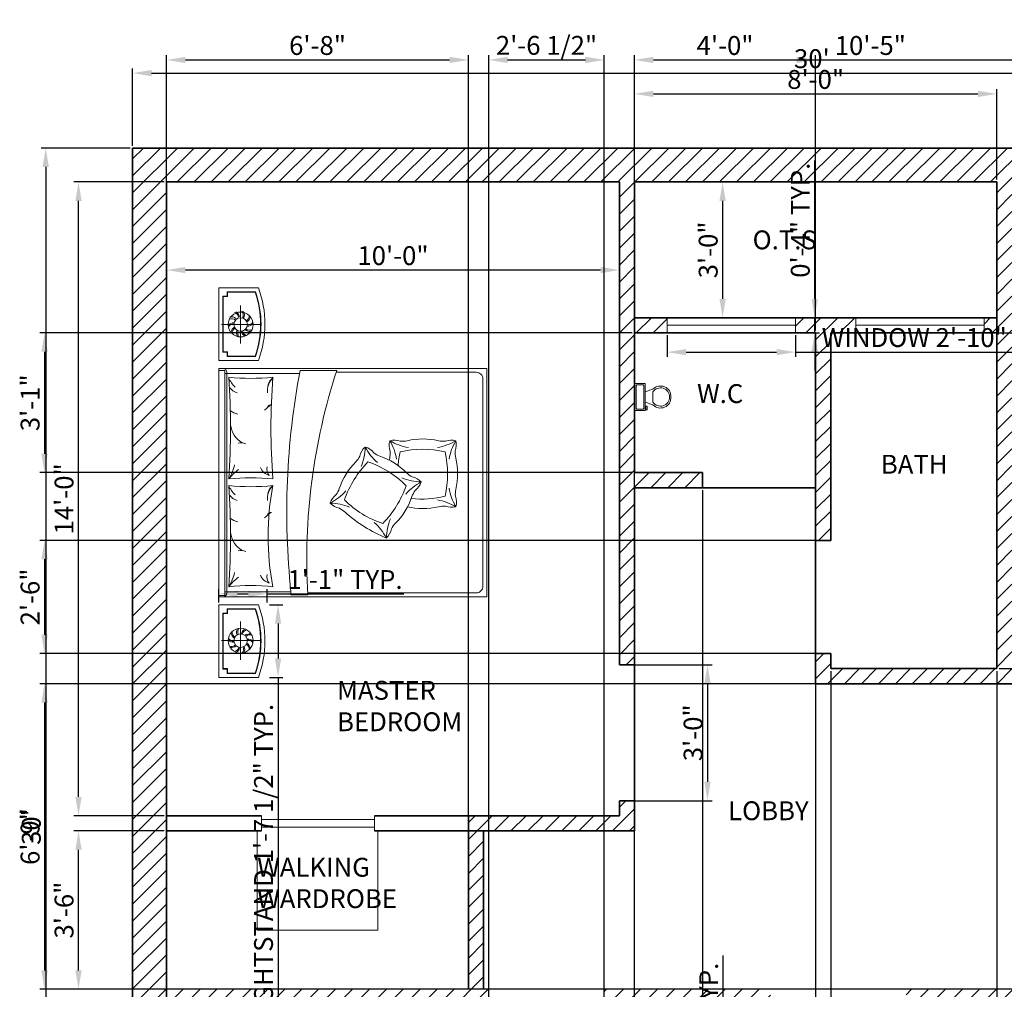
# Model space of a CAD drawing. Units: inches. Extents: x -33 to 381, y -443 to 47.
# Tile 4 of 5: x -33 to 228, y -210 to 47. Entities that reach past the tile are written whole.
import ezdxf

# ---------------------------------------------------------------- set-up
doc = ezdxf.new("R2010")
doc.units = ezdxf.units.IN
for name, color, linetype, lineweight in [('A-ANNO-DIMS', 2, 'Continuous', 18), ('A-AREA-IDEN', 7, 'Continuous', 18), ('A-DOOR', 4, 'Continuous', 18), ('A-FLOR-CASE', 9, 'Continuous', 18), ('A-FLOR-FIXT', 9, 'Continuous', 18), ('A-GLAZ', 4, 'Continuous', 18), ('A-WALL', 7, 'Continuous', 35), ('A-WALL-PATT', 251, 'Continuous', 13), ('furn', 8, 'Continuous', 13)]:
    doc.layers.add(name, color=color, linetype=linetype, lineweight=lineweight)
doc.styles.get("Standard").update_dxf_attribs({"font": 'arial.ttf'})
doc.dimstyles.new('ISO-25', dxfattribs={"dimtxt": 5, "dimasz": 5, "dimexe": 1.25, "dimexo": 0.625, "dimtad": 1, "dimlunit": 3, "dimtxsty": 'Standard', "dimcen": 2.5, "dimadec": 0, "dimazin": 0, "dimtfac": 1, "dimtmove": 0, "dimatfit": 3, "dimfxl": 1, "dimarcsym": 0})
pattern_1 = [(45, (-607.8963, -64.2963), (-2.245064, 2.245064), [])]

# ---------------------------------------------------------------- blocks, each defined once
blk = doc.blocks.new('*U7')
for p, q in [((9.5, -6), (9.5, -2)), ((-10, -8.5), (-8, -8.5)), ((-10, -9.5), (-10, -8.5)), ((-7, -9.5), (-10, -9.5)), ((-8, -8.5), (-8, -8)), ((-7, -8), (-7, -9.5)), ((-4, -8), (-6, -14)), ((4, -14), (-4, -14)), ((4, -8), (6, -14))]:
    blk.add_line(p, q)
blk.add_lwpolyline([(10.5, -8), (10.5, 0), (-10.5, 0), (-10.5, -8)], close=True)
for points in [[(-9.5, -2), (-9.5, -6)], [(8.5, -1), (-8.5, -1)], [(-8.5, -7), (8.5, -7)]]:
    blk.add_lwpolyline(points)
for centre, radius, start, end in [((-8.625, -1.875), 0.8839, 81.8699, 188.1301), ((-8.625, -6.125), 0.8839, 171.869898, 278.1301), ((8.625, -1.875), 0.8839, 351.8699, 98.1301), ((8.625, -6.125), 0.8839, 261.8699, 8.1301), ((-0.4772, -19.9188), 8.0953, 133.01722, 273.38), ((0.0374, -19.8731), 7.127, 124.50543, 269.7), ((-0.0373, -19.8731), 7.127, 270.3, 55.4946), ((0.4773, -19.9188), 8.0953, 266.62, 46.9828)]:
    blk.add_arc(centre, radius, start, end)
blk = doc.blocks.new('*D8')
at = {"layer": 'A-ANNO-DIMS', "color": 0, "lineweight": -2, "transparency": 16777216}
for p, q in [((-3.46, 13.8), (-3.46, 34.29)), ((356.54, 13.8), (356.54, 34.29)), ((1.54, 33.04), (351.54, 33.04))]:
    blk.add_line(p, q, dxfattribs=at)
at = {"layer": 'A-ANNO-DIMS', "color": 0, "transparency": 16777216}
for points in [[(1.54, 33.87), (1.54, 32.21), (-3.46, 33.04)], [(351.54, 33.87), (351.54, 32.21), (356.54, 33.04)]]:
    blk.add_solid(points, dxfattribs=at)
at = {"layer": 'Defpoints', "color": 0, "transparency": 16777216}
for p in [(356.54, 33.04), (-3.46, 13.18), (356.54, 13.18)]:
    blk.add_point(p, dxfattribs=at)
at = {"layer": 'A-ANNO-DIMS', "color": 0, "transparency": 16777216, "insert": (176.54, 36.22), "char_height": 5, "attachment_point": 5}
blk.add_mtext("30'", dxfattribs=at)
blk = doc.blocks.new('*D11')
at = {"layer": 'A-ANNO-DIMS', "color": 0, "lineweight": -2, "transparency": 16777216}
for p, q in [((-4.08, 13.18), (-27.74, 13.18)), ((-26.49, 8.18), (-26.49, -341.82)), ((4.92, -346.82), (-27.74, -346.82))]:
    blk.add_line(p, q, dxfattribs=at)
at = {"layer": 'A-ANNO-DIMS', "color": 0, "transparency": 16777216}
for points in [[(-27.33, 8.18), (-25.66, 8.18), (-26.49, 13.18)], [(-27.33, -341.82), (-25.66, -341.82), (-26.49, -346.82)]]:
    blk.add_solid(points, dxfattribs=at)
at = {"layer": 'Defpoints', "color": 0, "transparency": 16777216}
for p in [(-3.46, 13.18), (-26.49, -346.82), (5.54, -346.82)]:
    blk.add_point(p, dxfattribs=at)
at = {"layer": 'A-ANNO-DIMS', "color": 0, "transparency": 16777216, "insert": (-29.67, -166.82), "char_height": 5, "attachment_point": 5, "rotation": 90}
blk.add_mtext("30'", dxfattribs=at)
blk = doc.blocks.new('NIGHTSTAND-LARGE')
blk.add_lwpolyline([(10.5, 19.25), (0, 19.25), (0, 0), (10.5, 0, 0.181818)], format="xyb", close=True)
for points in [[(1.05, 16.94), (2.31, 16.94), (2.31, 18.2)], [(1.05, 17.05), (2.21, 17.05), (2.21, 18.2)], [(1.05, 17.05), (1.05, 2.21)], [(1.16, 17.05), (1.16, 2.21)], [(1.05, 2.31), (2.31, 2.31), (2.31, 1.05)], [(1.05, 2.21), (2.21, 2.21), (2.21, 1.05)]]:
    blk.add_lwpolyline(points)
for points in [[(2.21, 1.05), (9.77, 1.05, 0.167087), (9.77, 18.2), (2.21, 18.2)], [(2.21, 1.16), (9.69, 1.16, 0.165559), (9.69, 18.1), (2.21, 18.1)]]:
    blk.add_lwpolyline(points, format="xyb")
blk = doc.blocks.new('WINDOW-34IN')
blk.add_line((0, 2), (34, 2))
blk.add_lwpolyline([(0, 4), (34, 4), (34, 0), (0, 0)], close=True)
blk = doc.blocks.new('*D23')
at = {"layer": 'A-ANNO-DIMS', "color": 0, "lineweight": -2, "transparency": 16777216}
for p, q in [((32.82, -107.88), (36.33, -107.88)), ((35.08, -112.88), (35.08, -122.13)), ((32.82, -127.13), (36.33, -127.13)), ((35.08, -127.13), (35.08, -222.61))]:
    blk.add_line(p, q, dxfattribs=at)
at = {"layer": 'A-ANNO-DIMS', "color": 0, "transparency": 16777216}
for points in [[(34.24, -112.88), (35.91, -112.88), (35.08, -107.88)], [(34.24, -122.13), (35.91, -122.13), (35.08, -127.13)]]:
    blk.add_solid(points, dxfattribs=at)
at = {"layer": 'Defpoints', "color": 0, "transparency": 16777216}
for p in [(32.19, -107.88), (32.19, -127.13), (35.08, -127.13)]:
    blk.add_point(p, dxfattribs=at)
at = {"layer": 'A-ANNO-DIMS', "color": 0, "transparency": 16777216, "insert": (31.87, -177.37), "char_height": 5, "attachment_point": 5, "rotation": 90}
blk.add_mtext('NIGHTSTAND 1\'-7 1/2" TYP.', dxfattribs=at)
blk = doc.blocks.new('*D24')
at = {"layer": 'A-ANNO-DIMS', "color": 0, "lineweight": -2, "transparency": 16777216}
for p, q in [((19.36, -107.25), (19.36, -103.74)), ((32.19, -107.25), (32.19, -103.74)), ((24.36, -104.99), (27.19, -104.99)), ((32.19, -104.99), (68.45, -104.99))]:
    blk.add_line(p, q, dxfattribs=at)
at = {"layer": 'A-ANNO-DIMS', "color": 0, "transparency": 16777216}
for points in [[(24.36, -104.16), (24.36, -105.82), (19.36, -104.99)], [(27.19, -104.16), (27.19, -105.82), (32.19, -104.99)]]:
    blk.add_solid(points, dxfattribs=at)
at = {"layer": 'Defpoints', "color": 0, "transparency": 16777216}
for p in [(32.19, -104.99), (19.36, -107.88), (32.19, -107.88)]:
    blk.add_point(p, dxfattribs=at)
at = {"layer": 'A-ANNO-DIMS', "color": 0, "transparency": 16777216, "insert": (52.82, -101.85), "char_height": 5, "attachment_point": 5}
blk.add_mtext('1\'-1" TYP.', dxfattribs=at)
blk = doc.blocks.new('*D29')
at = {"layer": 'A-ANNO-DIMS', "color": 0, "lineweight": -2, "transparency": 16777216}
for p, q in [((138.2, -36.45), (138.2, -42.17)), ((172.2, -36.45), (172.2, -42.17)), ((143.2, -40.92), (167.2, -40.92)), ((172.2, -40.92), (245.61, -40.92))]:
    blk.add_line(p, q, dxfattribs=at)
at = {"layer": 'A-ANNO-DIMS', "color": 0, "transparency": 16777216}
for points in [[(143.2, -40.09), (143.2, -41.75), (138.2, -40.92)], [(167.2, -40.09), (167.2, -41.75), (172.2, -40.92)]]:
    blk.add_solid(points, dxfattribs=at)
at = {"layer": 'Defpoints', "color": 0, "transparency": 16777216}
for p in [(138.2, -35.82), (172.2, -35.82), (172.2, -40.92)]:
    blk.add_point(p, dxfattribs=at)
at = {"layer": 'A-ANNO-DIMS', "color": 0, "transparency": 16777216, "insert": (211.4, -37.71), "char_height": 5, "attachment_point": 5}
blk.add_mtext('WINDOW 2\'-10" TYP.', dxfattribs=at)
blk = doc.blocks.new('*D30')
at = {"layer": 'A-ANNO-DIMS', "color": 0, "lineweight": -2, "transparency": 16777216}
for p, q in [((177.3, -26.82), (177.3, 9.91)), ((172.83, -31.82), (178.55, -31.82)), ((177.3, -35.82), (177.3, -31.82)), ((172.83, -35.82), (178.55, -35.82)), ((177.3, -40.82), (177.3, -45.82))]:
    blk.add_line(p, q, dxfattribs=at)
at = {"layer": 'A-ANNO-DIMS', "color": 0, "transparency": 16777216}
for points in [[(176.47, -26.82), (178.13, -26.82), (177.3, -31.82)], [(176.47, -40.82), (178.13, -40.82), (177.3, -35.82)]]:
    blk.add_solid(points, dxfattribs=at)
at = {"layer": 'Defpoints', "color": 0, "transparency": 16777216}
for p in [(172.2, -31.82), (177.3, -31.82), (172.2, -35.82)]:
    blk.add_point(p, dxfattribs=at)
at = {"layer": 'A-ANNO-DIMS', "color": 0, "transparency": 16777216, "insert": (174.12, -5.96), "char_height": 5, "attachment_point": 5, "rotation": 90}
blk.add_mtext('0\'-4" TYP.', dxfattribs=at)
blk = doc.blocks.new('*D35')
at = {"layer": 'A-ANNO-DIMS', "color": 0, "lineweight": -2, "transparency": 16777216}
for p, q in [((153.06, -280.47), (153.06, -200.88)), ((153.04, -285.47), (154.31, -285.47)), ((153.06, -289.78), (153.06, -285.47)), ((153.04, -289.78), (154.31, -289.78)), ((153.06, -294.78), (153.06, -299.78))]:
    blk.add_line(p, q, dxfattribs=at)
at = {"layer": 'A-ANNO-DIMS', "color": 0, "transparency": 16777216}
for points in [[(152.22, -280.47), (153.89, -280.47), (153.06, -285.47)], [(152.22, -294.78), (153.89, -294.78), (153.06, -289.78)]]:
    blk.add_solid(points, dxfattribs=at)
at = {"layer": 'Defpoints', "color": 0, "transparency": 16777216}
for p in [(152.41, -285.47), (153.06, -285.47), (152.41, -289.78)]:
    blk.add_point(p, dxfattribs=at)
at = {"layer": 'A-ANNO-DIMS', "color": 0, "transparency": 16777216, "insert": (149.85, -238.18), "char_height": 5, "attachment_point": 5, "rotation": 90}
blk.add_mtext('BURNER 0\'-4 1/2" TYP.', dxfattribs=at)
blk = doc.blocks.new('*D40')
at = {"layer": 'A-ANNO-DIMS', "color": 0, "lineweight": -2, "transparency": 16777216}
for p, q in [((5.54, 3.55), (5.54, -20.42)), ((125.54, 3.55), (125.54, -20.42)), ((120.54, -19.17), (10.54, -19.17))]:
    blk.add_line(p, q, dxfattribs=at)
at = {"layer": 'A-ANNO-DIMS', "color": 0, "transparency": 16777216}
for points in [[(10.54, -18.34), (10.54, -20), (5.54, -19.17)], [(120.54, -18.34), (120.54, -20), (125.54, -19.17)]]:
    blk.add_solid(points, dxfattribs=at)
at = {"layer": 'Defpoints', "color": 0, "transparency": 16777216}
for p in [(5.54, 4.18), (125.54, 4.18), (5.54, -19.17)]:
    blk.add_point(p, dxfattribs=at)
at = {"layer": 'A-ANNO-DIMS', "color": 0, "transparency": 16777216, "insert": (65.54, -15.99), "char_height": 5, "attachment_point": 5}
blk.add_mtext('10\'-0"', dxfattribs=at)
blk = doc.blocks.new('*D41')
at = {"layer": 'A-ANNO-DIMS', "color": 0, "lineweight": -2, "transparency": 16777216}
for p, q in [((129.54, 4.8), (129.54, 28.78)), ((225.54, 4.8), (225.54, 28.78)), ((134.54, 27.53), (220.54, 27.53))]:
    blk.add_line(p, q, dxfattribs=at)
at = {"layer": 'A-ANNO-DIMS', "color": 0, "transparency": 16777216}
for points in [[(134.54, 28.36), (134.54, 26.7), (129.54, 27.53)], [(220.54, 28.36), (220.54, 26.7), (225.54, 27.53)]]:
    blk.add_solid(points, dxfattribs=at)
at = {"layer": 'Defpoints', "color": 0, "transparency": 16777216}
for p in [(225.54, 27.53), (129.54, 4.18), (225.54, 4.18)]:
    blk.add_point(p, dxfattribs=at)
at = {"layer": 'A-ANNO-DIMS', "color": 0, "transparency": 16777216, "insert": (177.54, 30.71), "char_height": 5, "attachment_point": 5}
blk.add_mtext('8\'-0"', dxfattribs=at)
blk = doc.blocks.new('*D43')
at = {"layer": 'A-ANNO-DIMS', "color": 0, "lineweight": -2, "transparency": 16777216}
for p, q in [((4.92, 4.18), (-19.06, 4.18)), ((-17.81, -158.82), (-17.81, -0.82)), ((4.92, -163.82), (-19.06, -163.82))]:
    blk.add_line(p, q, dxfattribs=at)
at = {"layer": 'A-ANNO-DIMS', "color": 0, "transparency": 16777216}
for points in [[(-18.64, -0.82), (-16.98, -0.82), (-17.81, 4.18)], [(-18.64, -158.82), (-16.98, -158.82), (-17.81, -163.82)]]:
    blk.add_solid(points, dxfattribs=at)
at = {"layer": 'Defpoints', "color": 0, "transparency": 16777216}
for p in [(-17.81, 4.18), (5.54, 4.18), (5.54, -163.82)]:
    blk.add_point(p, dxfattribs=at)
at = {"layer": 'A-ANNO-DIMS', "color": 0, "transparency": 16777216, "insert": (-20.99, -79.82), "char_height": 5, "attachment_point": 5, "rotation": 90}
blk.add_mtext('14\'-0"', dxfattribs=at)
blk = doc.blocks.new('*D44')
at = {"layer": 'A-ANNO-DIMS', "color": 0, "lineweight": -2, "transparency": 16777216}
for p, q in [((4.92, -167.82), (-19.06, -167.82)), ((-17.81, -204.82), (-17.81, -172.82)), ((4.92, -209.82), (-19.06, -209.82))]:
    blk.add_line(p, q, dxfattribs=at)
at = {"layer": 'A-ANNO-DIMS', "color": 0, "transparency": 16777216}
for points in [[(-18.64, -172.82), (-16.98, -172.82), (-17.81, -167.82)], [(-18.64, -204.82), (-16.98, -204.82), (-17.81, -209.82)]]:
    blk.add_solid(points, dxfattribs=at)
at = {"layer": 'Defpoints', "color": 0, "transparency": 16777216}
for p in [(-17.81, -167.82), (5.54, -167.82), (5.54, -209.82)]:
    blk.add_point(p, dxfattribs=at)
at = {"layer": 'A-ANNO-DIMS', "color": 0, "transparency": 16777216, "insert": (-20.99, -188.82), "char_height": 5, "attachment_point": 5, "rotation": 90}
blk.add_mtext('3\'-6"', dxfattribs=at)
blk = doc.blocks.new('*D46')
at = {"layer": 'A-ANNO-DIMS', "color": 0, "lineweight": -2, "transparency": 16777216}
for p, q in [((5.54, -209.2), (5.54, 37.78)), ((85.54, -209.2), (85.54, 37.78)), ((10.54, 36.53), (80.54, 36.53))]:
    blk.add_line(p, q, dxfattribs=at)
at = {"layer": 'A-ANNO-DIMS', "color": 0, "transparency": 16777216}
for points in [[(10.54, 37.36), (10.54, 35.7), (5.54, 36.53)], [(80.54, 37.36), (80.54, 35.7), (85.54, 36.53)]]:
    blk.add_solid(points, dxfattribs=at)
at = {"layer": 'Defpoints', "color": 0, "transparency": 16777216}
for p in [(85.54, 36.53), (5.54, -209.82), (85.54, -209.82)]:
    blk.add_point(p, dxfattribs=at)
at = {"layer": 'A-ANNO-DIMS', "color": 0, "transparency": 16777216, "insert": (45.54, 39.71), "char_height": 5, "attachment_point": 5}
blk.add_mtext('6\'-8"', dxfattribs=at)
blk = doc.blocks.new('*D47')
at = {"layer": 'A-ANNO-DIMS', "color": 0, "lineweight": -2, "transparency": 16777216}
for p, q in [((129.54, -218.2), (129.54, 37.78)), ((254.54, -218.2), (254.54, 37.78)), ((134.54, 36.53), (249.54, 36.53))]:
    blk.add_line(p, q, dxfattribs=at)
at = {"layer": 'A-ANNO-DIMS', "color": 0, "transparency": 16777216}
for points in [[(134.54, 37.36), (134.54, 35.7), (129.54, 36.53)], [(249.54, 37.36), (249.54, 35.7), (254.54, 36.53)]]:
    blk.add_solid(points, dxfattribs=at)
at = {"layer": 'Defpoints', "color": 0, "transparency": 16777216}
for p in [(254.54, 36.53), (129.54, -218.82), (254.54, -218.82)]:
    blk.add_point(p, dxfattribs=at)
at = {"layer": 'A-ANNO-DIMS', "color": 0, "transparency": 16777216, "insert": (192.04, 39.71), "char_height": 5, "attachment_point": 5}
blk.add_mtext('10\'-5"', dxfattribs=at)
blk = doc.blocks.new('*D50')
at = {"layer": 'A-ANNO-DIMS', "color": 0, "lineweight": -2, "transparency": 16777216}
for p, q in [((130.17, 4.18), (154.14, 4.18)), ((152.89, -0.82), (152.89, -26.82)), ((130.17, -31.82), (154.14, -31.82))]:
    blk.add_line(p, q, dxfattribs=at)
at = {"layer": 'A-ANNO-DIMS', "color": 0, "transparency": 16777216}
for points in [[(152.06, -0.82), (153.72, -0.82), (152.89, 4.18)], [(152.06, -26.82), (153.72, -26.82), (152.89, -31.82)]]:
    blk.add_solid(points, dxfattribs=at)
at = {"layer": 'Defpoints', "color": 0, "transparency": 16777216}
for p in [(129.54, 4.18), (129.54, -31.82), (152.89, -31.82)]:
    blk.add_point(p, dxfattribs=at)
at = {"layer": 'A-ANNO-DIMS', "color": 0, "transparency": 16777216, "insert": (149.71, -13.82), "char_height": 5, "attachment_point": 5, "rotation": 90}
blk.add_mtext('3\'-0"', dxfattribs=at)
blk = doc.blocks.new('*D51')
at = {"layer": 'A-ANNO-DIMS', "color": 0, "lineweight": -2, "transparency": 16777216}
for p, q in [((129.54, -35.2), (129.54, 37.78)), ((177.54, -35.2), (177.54, 37.78)), ((134.54, 36.53), (172.54, 36.53))]:
    blk.add_line(p, q, dxfattribs=at)
at = {"layer": 'A-ANNO-DIMS', "color": 0, "transparency": 16777216}
for points in [[(134.54, 37.36), (134.54, 35.7), (129.54, 36.53)], [(172.54, 37.36), (172.54, 35.7), (177.54, 36.53)]]:
    blk.add_solid(points, dxfattribs=at)
at = {"layer": 'Defpoints', "color": 0, "transparency": 16777216}
for p in [(177.54, 36.53), (129.54, -35.82), (177.54, -35.82)]:
    blk.add_point(p, dxfattribs=at)
at = {"layer": 'A-ANNO-DIMS', "color": 0, "transparency": 16777216, "insert": (153.54, 39.71), "char_height": 5, "attachment_point": 5}
blk.add_mtext('4\'-0"', dxfattribs=at)
blk = doc.blocks.new('*D52')
at = {"layer": 'A-ANNO-DIMS', "color": 0, "lineweight": -2, "transparency": 16777216}
for p, q in [((181.54, -125.45), (181.54, -443.26)), ((225.54, -125.45), (225.54, -443.26)), ((186.54, -442.01), (220.54, -442.01))]:
    blk.add_line(p, q, dxfattribs=at)
at = {"layer": 'A-ANNO-DIMS', "color": 0, "transparency": 16777216}
for points in [[(186.54, -441.18), (186.54, -442.84), (181.54, -442.01)], [(220.54, -441.18), (220.54, -442.84), (225.54, -442.01)]]:
    blk.add_solid(points, dxfattribs=at)
at = {"layer": 'Defpoints', "color": 0, "transparency": 16777216}
for p in [(181.54, -124.82), (225.54, -124.82), (225.54, -442.01)]:
    blk.add_point(p, dxfattribs=at)
at = {"layer": 'A-ANNO-DIMS', "color": 0, "transparency": 16777216, "insert": (203.54, -438.83), "char_height": 5, "attachment_point": 5}
blk.add_mtext('3\'-8"', dxfattribs=at)
blk = doc.blocks.new('*D53')
at = {"layer": 'A-ANNO-DIMS', "color": 0, "lineweight": -2, "transparency": 16777216}
for p, q in [((128.92, -35.82), (-28.06, -35.82)), ((-26.81, -40.82), (-26.81, -67.86)), ((128.92, -72.86), (-28.06, -72.86))]:
    blk.add_line(p, q, dxfattribs=at)
at = {"layer": 'A-ANNO-DIMS', "color": 0, "transparency": 16777216}
for points in [[(-27.64, -40.82), (-25.98, -40.82), (-26.81, -35.82)], [(-27.64, -67.86), (-25.98, -67.86), (-26.81, -72.86)]]:
    blk.add_solid(points, dxfattribs=at)
at = {"layer": 'Defpoints', "color": 0, "transparency": 16777216}
for p in [(129.54, -35.82), (-26.81, -72.86), (129.54, -72.86)]:
    blk.add_point(p, dxfattribs=at)
at = {"layer": 'A-ANNO-DIMS', "color": 0, "transparency": 16777216, "insert": (-29.99, -54.34), "char_height": 5, "attachment_point": 5, "rotation": 90}
blk.add_mtext('3\'-1"', dxfattribs=at)
blk = doc.blocks.new('*D54')
at = {"layer": 'A-ANNO-DIMS', "color": 0, "lineweight": -2, "transparency": 16777216}
for p, q in [((226.17, -35.82), (381.14, -35.82)), ((379.89, -40.82), (379.89, -119.82)), ((226.17, -124.82), (381.14, -124.82))]:
    blk.add_line(p, q, dxfattribs=at)
at = {"layer": 'A-ANNO-DIMS', "color": 0, "transparency": 16777216}
for points in [[(379.06, -40.82), (380.72, -40.82), (379.89, -35.82)], [(379.06, -119.82), (380.72, -119.82), (379.89, -124.82)]]:
    blk.add_solid(points, dxfattribs=at)
at = {"layer": 'Defpoints', "color": 0, "transparency": 16777216}
for p in [(225.54, -35.82), (225.54, -124.82), (379.89, -124.82)]:
    blk.add_point(p, dxfattribs=at)
at = {"layer": 'A-ANNO-DIMS', "color": 0, "transparency": 16777216, "insert": (376.72, -80.32), "char_height": 5, "attachment_point": 5, "rotation": 90}
blk.add_mtext('7\'-5"', dxfattribs=at)
blk = doc.blocks.new('*D57')
at = {"layer": 'A-ANNO-DIMS', "color": 0, "lineweight": -2, "transparency": 16777216}
for p, q in [((253.92, -128.82), (-28.06, -128.82)), ((-26.81, -133.82), (-26.81, -204.82)), ((253.92, -209.82), (-28.06, -209.82))]:
    blk.add_line(p, q, dxfattribs=at)
at = {"layer": 'A-ANNO-DIMS', "color": 0, "transparency": 16777216}
for points in [[(-27.64, -133.82), (-25.98, -133.82), (-26.81, -128.82)], [(-27.64, -204.82), (-25.98, -204.82), (-26.81, -209.82)]]:
    blk.add_solid(points, dxfattribs=at)
at = {"layer": 'Defpoints', "color": 0, "transparency": 16777216}
for p in [(254.54, -128.82), (-26.81, -209.82), (254.54, -209.82)]:
    blk.add_point(p, dxfattribs=at)
at = {"layer": 'A-ANNO-DIMS', "color": 0, "transparency": 16777216, "insert": (-29.99, -169.32), "char_height": 5, "attachment_point": 5, "rotation": 90}
blk.add_mtext('6\'-9"', dxfattribs=at)
blk = doc.blocks.new('*D61')
at = {"layer": 'A-ANNO-DIMS', "color": 0, "lineweight": -2, "transparency": 16777216}
for p, q in [((147.54, -77.49), (147.54, -443.26)), ((177.54, -77.49), (177.54, -443.26)), ((152.54, -442.01), (172.54, -442.01))]:
    blk.add_line(p, q, dxfattribs=at)
at = {"layer": 'A-ANNO-DIMS', "color": 0, "transparency": 16777216}
for points in [[(152.54, -441.18), (152.54, -442.84), (147.54, -442.01)], [(172.54, -441.18), (172.54, -442.84), (177.54, -442.01)]]:
    blk.add_solid(points, dxfattribs=at)
at = {"layer": 'Defpoints', "color": 0, "transparency": 16777216}
for p in [(147.54, -76.86), (177.54, -76.86), (177.54, -442.01)]:
    blk.add_point(p, dxfattribs=at)
at = {"layer": 'A-ANNO-DIMS', "color": 0, "transparency": 16777216, "insert": (162.54, -438.83), "char_height": 5, "attachment_point": 5}
blk.add_mtext('2\'-6"', dxfattribs=at)
blk = doc.blocks.new('*D62')
at = {"layer": 'A-ANNO-DIMS', "color": 0, "lineweight": -2, "transparency": 16777216}
for p, q in [((180.92, -90.82), (-28.06, -90.82)), ((-26.81, -95.82), (-26.81, -115.82)), ((180.92, -120.82), (-28.06, -120.82))]:
    blk.add_line(p, q, dxfattribs=at)
at = {"layer": 'A-ANNO-DIMS', "color": 0, "transparency": 16777216}
for points in [[(-27.64, -95.82), (-25.98, -95.82), (-26.81, -90.82)], [(-27.64, -115.82), (-25.98, -115.82), (-26.81, -120.82)]]:
    blk.add_solid(points, dxfattribs=at)
at = {"layer": 'Defpoints', "color": 0, "transparency": 16777216}
for p in [(181.54, -90.82), (-26.81, -120.82), (181.54, -120.82)]:
    blk.add_point(p, dxfattribs=at)
at = {"layer": 'A-ANNO-DIMS', "color": 0, "transparency": 16777216, "insert": (-29.99, -105.82), "char_height": 5, "attachment_point": 5, "rotation": 90}
blk.add_mtext('2\'-6"', dxfattribs=at)
blk = doc.blocks.new('*D64')
at = {"layer": 'A-ANNO-DIMS', "color": 0, "lineweight": -2, "transparency": 16777216}
for p, q in [((90.91, -218.2), (90.91, 37.78)), ((121.54, -218.2), (121.54, 37.78)), ((95.91, 36.53), (116.54, 36.53))]:
    blk.add_line(p, q, dxfattribs=at)
at = {"layer": 'A-ANNO-DIMS', "color": 0, "transparency": 16777216}
for points in [[(95.91, 37.36), (95.91, 35.7), (90.91, 36.53)], [(116.54, 37.36), (116.54, 35.7), (121.54, 36.53)]]:
    blk.add_solid(points, dxfattribs=at)
at = {"layer": 'Defpoints', "color": 0, "transparency": 16777216}
for p in [(121.54, 36.53), (90.91, -218.82), (121.54, -218.82)]:
    blk.add_point(p, dxfattribs=at)
at = {"layer": 'A-ANNO-DIMS', "color": 0, "transparency": 16777216, "insert": (106.22, 39.74), "char_height": 5, "attachment_point": 5}
blk.add_mtext('2\'-6 1/2"', dxfattribs=at)
blk = doc.blocks.new('*D65')
at = {"layer": 'A-ANNO-DIMS', "color": 0, "lineweight": -2, "transparency": 16777216}
for p, q in [((126.17, -123.82), (150.14, -123.82)), ((148.89, -128.82), (148.89, -154.82)), ((126.17, -159.82), (150.14, -159.82))]:
    blk.add_line(p, q, dxfattribs=at)
at = {"layer": 'A-ANNO-DIMS', "color": 0, "transparency": 16777216}
for points in [[(148.06, -128.82), (149.72, -128.82), (148.89, -123.82)], [(148.06, -154.82), (149.72, -154.82), (148.89, -159.82)]]:
    blk.add_solid(points, dxfattribs=at)
at = {"layer": 'Defpoints', "color": 0, "transparency": 16777216}
for p in [(125.54, -123.82), (125.54, -159.82), (148.89, -159.82)]:
    blk.add_point(p, dxfattribs=at)
at = {"layer": 'A-ANNO-DIMS', "color": 0, "transparency": 16777216, "insert": (145.71, -141.82), "char_height": 5, "attachment_point": 5, "rotation": 90}
blk.add_mtext('3\'-0"', dxfattribs=at)

msp = doc.modelspace()

# ---------------------------------------------------------------- hatches: boundary and pattern name
at = {"layer": 'A-WALL-PATT'}
h = msp.add_hatch(dxfattribs=at)
h.set_pattern_fill('ANSI31', color=256)
h.set_pattern_definition(pattern_1)
h.paths.add_polyline_path([(356.541, 13.18), (-3.459, 13.18), (-3.459, -346.82), (-3.459, -382.82), (254.541, -382.82), (254.541, -378.82), (5.541, -378.82), (5.541, -346.82), (36.25, -346.82), (36.25, -337.82), (5.541, -337.82), (5.541, 4.18), (125.541, 4.18), (125.541, -123.82), (129.541, -123.82), (129.541, -76.862), (147.541, -76.862), (147.541, -72.862), (129.541, -72.862), (129.541, 4.18), (225.541, 4.18), (225.541, -124.82), (181.541, -124.82), (181.541, -120.82), (177.541, -120.82), (177.541, -128.82), (229.541, -128.82), (229.541, 4.18), (347.541, 4.18), (347.541, -119.82), (329.098, -119.82), (329.098, -128.82), (347.541, -128.82), (347.541, -373.82), (343.541, -373.82), (343.541, -382.82), (356.541, -382.82), (356.541, -346.82)])
h.paths.add_polyline_path([(181.541, -35.82), (188.17, -35.82), (188.17, -31.82), (172.2, -31.82), (172.2, -35.82), (177.541, -35.82), (177.541, -90.82), (181.541, -90.82)], flags=17)
h.paths.add_polyline_path([(225.541, -31.82), (222.17, -31.82), (222.17, -35.82), (225.541, -35.82)], flags=17)
h.paths.add_polyline_path([(138.2, -31.82), (129.541, -31.82), (129.541, -35.82), (138.2, -35.82)], flags=17)
h.paths.add_polyline_path([(89.541, -167.82), (85.541, -167.82), (85.541, -209.82), (5.541, -209.82), (5.541, -218.82), (90.906, -218.82), (90.906, -209.82), (89.541, -209.82)], flags=17)
h.paths.add_polyline_path([(165.541, -209.82), (125.541, -209.82), (121.541, -209.82), (121.541, -218.82), (125.541, -218.82), (125.541, -310.82), (160.374, -310.82), (160.374, -301.82), (129.541, -301.82), (129.541, -218.82), (165.541, -218.82)], flags=17)
h.paths.add_polyline_path([(263.541, -209.82), (254.541, -209.82), (201.541, -209.82), (201.541, -218.82), (254.541, -218.82), (254.541, -301.82), (214.374, -301.82), (214.374, -310.82), (254.541, -310.82), (263.541, -310.82)], flags=17)
h.paths.add_polyline_path([(263.541, -128.82), (275.098, -128.82), (275.098, -119.82), (254.541, -119.82), (254.541, -128.82), (254.541, -165.974), (263.541, -165.974)], flags=17)
h.paths.add_polyline_path([(263.541, -373.82), (254.541, -373.82), (254.541, -382.82), (263.541, -382.82)], flags=17)
h = msp.add_hatch(dxfattribs=at)
h.set_pattern_fill('ANSI31', color=256)
h.set_pattern_definition(pattern_1)
h.paths.add_polyline_path([(129.541, -159.82), (125.541, -159.82), (125.541, -163.82), (85.541, -163.82), (85.541, -167.82), (125.541, -167.82), (129.541, -167.82)])

# ---------------------------------------------------------------- linework, layer by layer
at = {"layer": 'A-DOOR'}
for p, q in [((30.717, -167.82), (30.717, -163.82)), ((60.656, -167.82), (60.656, -163.82)), ((30.717, -164.82), (60.656, -164.82)), ((30.717, -166.82), (60.656, -166.82))]:
    msp.add_line(p, q, dxfattribs=at)
at = {"layer": 'A-FLOR-CASE'}
for p, q in [((29.541, -167.82), (29.541, -194.142)), ((61.541, -167.82), (61.541, -194.142)), ((61.541, -194.142), (29.541, -194.142))]:
    msp.add_line(p, q, dxfattribs=at)
at = {"layer": 'A-WALL'}
for p, q in [((-3.459, -346.82), (-3.459, 13.18)), ((-3.459, 13.18), (356.541, 13.18)), ((5.541, -337.82), (5.541, 4.18)), ((5.541, 4.18), (125.541, 4.18)), ((125.541, -123.82), (125.541, 4.18)), ((129.541, 4.18), (225.541, 4.18)), ((129.541, -72.862), (129.541, 4.18)), ((225.541, -124.82), (225.541, 4.18)), ((129.541, -31.82), (225.541, -31.82)), ((129.541, -35.82), (177.541, -35.82)), ((177.541, -35.82), (177.541, -128.82)), ((181.541, -35.82), (181.541, -90.82)), ((181.541, -35.82), (225.541, -35.82)), ((147.541, -72.862), (129.541, -72.862)), ((147.541, -72.862), (147.541, -76.862)), ((129.541, -167.82), (129.541, -76.862)), ((177.541, -76.862), (129.541, -76.862)), ((181.541, -90.82), (177.541, -90.82)), ((181.541, -120.82), (177.541, -120.82)), ((181.541, -120.82), (181.541, -124.82)), ((125.541, -123.82), (129.541, -123.82)), ((225.541, -124.82), (181.541, -124.82)), ((229.541, -128.82), (177.541, -128.82)), ((125.541, -159.82), (129.541, -159.82)), ((125.541, -163.82), (125.541, -159.82)), ((5.541, -163.82), (30.717, -163.82)), ((60.656, -163.82), (125.541, -163.82)), ((85.541, -168.724), (85.541, -163.82)), ((5.541, -167.82), (30.717, -167.82)), ((60.656, -167.82), (125.541, -167.82)), ((85.541, -167.82), (85.541, -209.82)), ((89.541, -167.82), (89.541, -209.82)), ((125.541, -167.82), (129.541, -167.82))]:
    msp.add_line(p, q, dxfattribs=at)
at = {"layer": 'furn'}
for p, q in [((25.154, -28.555), (25.154, -38.649)), ((30.202, -33.602), (20.107, -33.602)), ((20.993, -46.613), (40.749, -46.613)), ((21.515, -104.728), (21.515, -46.278)), ((20.993, -104.429), (38.476, -104.429)), ((25.153, -122.451), (25.153, -112.357)), ((30.201, -117.404), (20.106, -117.404))]:
    msp.add_line(p, q, dxfattribs=at)
for points in [[(19.352, -105.778), (90.403, -105.778), (90.403, -45.228), (19.352, -45.228)], [(19.352, -45.793), (20.993, -45.793), (20.993, -105.428), (19.352, -105.428), (19.352, -45.228)]]:
    msp.add_lwpolyline(points, dxfattribs=at)
for points in [[(38.476, -105.249), (38.476, -104.429, -0.0729439), (40.919, -45.793), (50.627, -45.793, 0.0925678), (42.929, -105.249)], [(33.694, -74.551, 0.0585956), (21.997, -74.551, 0.0366479), (21.997, -47.574, 0.052163), (33.694, -47.574, 0.0369674)], [(33.694, -103.094, 0.0585956), (21.997, -103.094, 0.0368889), (21.997, -76.293, 0.052163), (33.694, -76.293, 0.0931113)]]:
    msp.add_lwpolyline(points, format="xyb", close=True, dxfattribs=at)
for points in [[(42.898, -104.728), (87.603, -104.728, 0.4142136), (89.353, -102.978), (89.353, -48.028, 0.4142136), (87.603, -46.278), (50.454, -46.278)], [(82.201, -64.399, 0.1594612), (79.445, -64.52, -0.0762829), (77.605, -64.399, 0.1150751), (69.298, -64.399, -0.0762829), (67.458, -64.52, 0.1594612), (64.701, -64.399)], [(66.494, -69.319, 0.0912961), (64.701, -64.399, 0.0912961), (69.616, -66.208, 0.0912961)], [(77.287, -66.208, 0.0912961), (82.201, -64.399, 0.0912961), (80.409, -69.319)], [(57.094, -71.208, 0.0912961), (58.174, -66.084, 0.0912961), (61.388, -70.218, 0.0912961)], [(73.027, -75.339, 0.1594612), (70.623, -73.984, -0.0762829), (69.126, -72.908, 0.1150751), (62.075, -68.515, -0.0762829), (60.45, -67.645, 0.1594612), (58.174, -66.084)], [(79.344, -79.138, 0.1110065), (79.333, -67.365, 0.1195491), (67.415, -67.365, 0.0332124), (66.865, -70.985)], [(62.807, -86.337, 0.1110065), (69.024, -76.339, 0.1195491), (58.909, -70.037, 0.1078134), (52.666, -80.004)], [(67.9, -74.275, 0.0912961), (73.027, -75.339, 0.0912961), (68.903, -78.567)], [(54.047, -82.001, 0.0912961), (48.919, -80.937, 0.0912961), (53.043, -77.709, 0.0912961)], [(80.409, -76.979, 0.0912961), (82.201, -81.899, 0.0912961), (77.287, -80.09, 0.0912961)], [(52.678, -80.058, 0.1218652), (62.807, -86.337, 0.1218652)], [(64.853, -85.068, 0.0912961), (63.772, -90.192, 0.0912961), (60.558, -86.058, 0.0912961)]]:
    msp.add_lwpolyline(points, format="xyb", dxfattribs=at)
for centre, radius in [((25.154, -33.602), 3.297), ((25.154, -33.602), 1.786), ((25.153, -117.404), 3.297), ((25.153, -117.404), 1.786)]:
    msp.add_circle(centre, radius, dxfattribs=at)
for centre, radius, start, end in [((23.053, -32.006), 1.616, 13.46198, 73.69983), ((22.894, -32.146), 2.118, 15.51025, 61.82997), ((24.234, -31.083), 1.616, 337.46198, 37.69983), ((24.023, -31.103), 2.118, 339.51025, 25.82997), ((25.822, -31.271), 1.616, 301.46198, 1.69983), ((23.328, -35.29), 2.118, 87.51025, 133.82997), ((23.244, -35.096), 1.616, 85.46198, 145.69983), ((22.731, -33.687), 1.616, 49.46198, 109.69983), ((22.594, -33.654), 2.118, 51.51025, 97.82997), ((25.64, -31.163), 2.118, 303.51025, 349.82997), ((26.981, -31.914), 2.118, 267.51025, 313.82997), ((27.065, -32.108), 1.616, 265.46198, 325.69983), ((24.669, -36.041), 2.118, 123.51025, 169.82997), ((24.487, -35.933), 1.616, 121.46198, 181.69983), ((26.195, -35.861), 2.118, 159.51025, 205.82997), ((25.985, -35.881), 1.616, 157.46198, 217.69983), ((27.324, -34.817), 2.118, 195.51025, 241.82997), ((27.165, -34.957), 1.616, 193.46198, 253.69983), ((27.624, -33.31), 2.118, 231.51025, 277.82997), ((27.578, -33.517), 1.616, 229.46198, 289.69983), ((20.465, -46.278), 1.05, 0, 90), ((30.014, -44.072), 8.821, 204.64565, 224.15848), ((37.041, -51.167), 4.783, 134.40604, 186.83423), ((35.372, -50.274), 3.031, 123.63488, 180.84559), ((25.889, -47.126), 4.896, 220.53543, 250.35581), ((25.244, -52.88), 4.55, 231.81741, 259.89867), ((41.829, -66.664), 14.612, 126.20852, 135.08491), ((33.197, -55.854), 0.981, 83.75428, 167.21866), ((28.933, -59.44), 6.488, 186.68493, 238.3182), ((25.323, -67.861), 2.907, 65.89274, 106.11919), ((68.584, -65.706), 4.097, 161.39955, 201.57741), ((77.242, -65.479), 5.076, 340.70232, 12.28404), ((60.779, -69.247), 4.097, 129.47264, 169.6505), ((58.722, -67.758), 6.077, 347.69876, 5.14771), ((88.088, -67.662), 6.077, 175.2252, 192.67415), ((68.638, -82.913), 18.287, 135.13065, 161.38844), ((51.323, -65.773), 6.077, 315.77185, 333.2208), ((82.482, -73.148), 18.287, 167.05756, 168.7033), ((64.364, -73.207), 18.287, 347.05756, 13.31535), ((12.218, -68.331), 11.59, 327.53791, 347.5233), ((32.935, -83.321), 14.019, 126.49353, 141.27919), ((33.963, -69.944), 3.889, 204.2916, 250.9896), ((34.776, -71.963), 2.66, 166.48229, 218.55627), ((68.247, -73.633), 5.076, 308.77541, 340.35713), ((30.014, -72.615), 8.821, 204.64565, 224.15848), ((37.041, -79.71), 4.783, 134.40604, 186.83423), ((35.372, -78.816), 3.031, 123.63488, 180.84559), ((45.571, -75.073), 6.077, 323.29829, 340.74724), ((76.297, -81.222), 6.077, 143.29829, 160.74724), ((88.124, -78.598), 6.077, 167.69876, 185.14771), ((25.889, -75.668), 4.896, 220.53543, 250.35581), ((53.036, -82.11), 4.281, 127.29372, 164.09733), ((53.23, -73.382), 18.287, 315.13065, 341.38844), ((73.329, -55.068), 24.809, 263.19556, 284.02838), ((77.925, -80.72), 4.436, 344.57915, 20.81985), ((41.829, -95.206), 14.612, 126.20852, 135.08491), ((33.197, -84.397), 0.981, 83.75428, 167.21866), ((52.192, -77.942), 4.436, 222.46578, 258.70648), ((48.568, -87.708), 6.077, 45.58539, 63.03435), ((78.276, -54.715), 38.327, 228.38179, 247.76439), ((73.451, -64.09), 18.287, 256.87111, 283.12889), ((78.919, -87.832), 6.077, 85.03874, 102.4877), ((81.008, -77.627), 4.436, 249.36661, 285.60731), ((25.244, -81.423), 4.55, 231.81741, 259.89867), ((60.767, -86.929), 4.436, 312.65224, 348.89294), ((70.545, -90.522), 6.077, 135.77185, 153.2208), ((28.933, -87.983), 6.488, 186.68493, 238.3182), ((25.323, -96.404), 2.907, 65.89274, 106.11919), ((12.218, -96.873), 11.59, 327.53791, 347.5233), ((32.935, -111.864), 14.019, 126.49353, 141.27919), ((33.963, -98.487), 3.889, 204.2916, 250.9896), ((34.776, -100.506), 2.66, 166.48229, 218.55627), ((20.465, -104.728), 1.05, 270, 0), ((26.194, -115.145), 2.118, 154.17003, 200.48975), ((25.984, -115.125), 1.616, 142.30017, 202.53802), ((27.323, -116.189), 2.118, 118.17003, 164.48975), ((27.164, -116.049), 1.616, 106.30017, 166.53802), ((23.327, -115.716), 2.118, 226.17003, 272.48975), ((23.243, -115.91), 1.616, 214.30017, 274.53802), ((24.668, -114.965), 2.118, 190.17003, 236.48975), ((24.486, -115.073), 1.616, 178.30017, 238.53802), ((27.623, -117.696), 2.118, 82.17003, 128.48975), ((27.577, -117.489), 1.616, 70.30017, 130.53802), ((26.98, -119.092), 2.118, 46.17003, 92.48975), ((27.064, -118.898), 1.616, 34.30017, 94.53802), ((22.73, -117.319), 1.616, 250.30017, 310.53802), ((22.684, -117.112), 2.118, 262.17003, 308.48975), ((23.143, -118.759), 1.616, 286.30017, 346.53802), ((22.984, -118.619), 2.118, 298.17003, 344.48975), ((24.323, -119.683), 1.616, 322.30017, 22.53802), ((24.113, -119.663), 2.118, 334.17003, 20.48975), ((25.821, -119.735), 1.616, 358.30017, 58.53802), ((25.639, -119.843), 2.118, 10.17003, 56.48975)]:
    msp.add_arc(centre, radius, start, end, dxfattribs=at)

# ---------------------------------------------------------------- block references
at = {"layer": 'A-FLOR-FIXT', "xscale": 0.3408667621120802, "yscale": 0.3408667621120802, "zscale": 0.3408667621120802, "rotation": 90}
msp.add_blockref('*U7', (129.64, -52.823), dxfattribs=at)
at = {"layer": 'A-GLAZ'}
for p in [(138.2, -35.82), (188.17, -35.82)]:
    msp.add_blockref('WINDOW-34IN', p, dxfattribs=at)
at = {"layer": 'furn'}
msp.add_blockref('NIGHTSTAND-LARGE', (19.353, -43.128), dxfattribs=at)
at = {"layer": 'furn', "extrusion": (0, 0, -1), "zscale": -1, "rotation": 180.0000065579598}
msp.add_blockref('NIGHTSTAND-LARGE', (-19.357, -107.878), dxfattribs=at)

# ---------------------------------------------------------------- texts
at = {"layer": 'A-AREA-IDEN', "char_height": 5, "attachment_point": 1}
for s, width, insert in [('O.T.S', 63.09937, (160.832, -8.669)), ('W.C', 21.72945, (146.122, -49.412)), ('BATH', 8.29008, (194.826, -68.149)), ('MASTER BEDROOM', 47.9251, (50.715, -128.063)), ('LOBBY', 67.77808, (154.344, -159.987)), ('WALKING\\PWARDROBE', 43.19295, (29.541, -174.965))]:
    msp.add_mtext_dynamic_manual_height_columns(s, width=width, gutter_width=12.5, heights=[0], dxfattribs=dict(at, insert=insert))

# ---------------------------------------------------------------- dimensions: what is measured, and where the dimension line sits
at = {"layer": 'A-ANNO-DIMS'}
for base, p1, p2, override, picture, middle in [((121.541, 36.53), (90.906, -218.82), (121.541, -218.82), {"dimdec": 1, "dimlfac": 1, "dimrnd": 0, "dimzin": 1, "dimdsep": 46, "dimlunit": 4, "dimfrac": 2}, '*D64', (106.224, 39.74)), ((85.541, 36.53), (5.541, -209.82), (85.541, -209.82), {"dimdec": 1, "dimlfac": 1, "dimrnd": 0, "dimzin": 1, "dimdsep": 46, "dimlunit": 4, "dimfrac": 2}, '*D46', (45.541, 39.708)), ((254.541, 36.53), (129.541, -218.82), (254.541, -218.82), {"dimdec": 1, "dimlfac": 1, "dimrnd": 0, "dimzin": 1, "dimdsep": 46, "dimlunit": 4, "dimfrac": 2}, '*D47', (192.041, 39.708)), ((177.541, 36.53), (129.541, -35.82), (177.541, -35.82), {"dimdec": 1, "dimlfac": 1, "dimrnd": 0, "dimzin": 1, "dimdsep": 46, "dimlunit": 4, "dimfrac": 2}, '*D51', (153.541, 39.708)), ((356.541, 33.041), (-3.459, 13.18), (356.541, 13.18), {"dimclrd": 0, "dimclre": 0, "dimclrt": 0}, '*D8', (176.541, 36.221)), ((177.541, -442.009), (147.541, -76.862), (177.541, -76.862), {"dimdec": 1, "dimlfac": 1, "dimrnd": 0, "dimzin": 1, "dimdsep": 46, "dimlunit": 4, "dimfrac": 2}, '*D61', (162.541, -438.832)), ((225.541, -442.009), (181.541, -124.82), (225.541, -124.82), {"dimdec": 1, "dimlfac": 1, "dimrnd": 0, "dimzin": 1, "dimdsep": 46, "dimlunit": 4, "dimfrac": 2}, '*D52', (203.541, -438.83))]:
    dim = msp.add_linear_dim(base=base, p1=p1, p2=p2, dimstyle='ISO-25', override=override, dxfattribs=at)
    dim.commit()
    dim.dimension.update_dxf_attribs({"geometry": picture, "text_midpoint": middle})
for base, p1, p2, angle, override, picture, middle in [((225.541, 27.53), (129.541, 4.18), (225.541, 4.18), 0, {"dimdec": 1, "dimlfac": 1, "dimrnd": 0, "dimzin": 1, "dimdsep": 46, "dimlunit": 4, "dimfrac": 2}, '*D41', (177.541, 30.708)), ((-26.493, -346.82), (-3.459, 13.18), (5.541, -346.82), 90, {"dimclrd": 0, "dimclre": 0, "dimclrt": 0}, '*D11', (-29.673, -166.82)), ((-17.809, 4.18), (5.541, -163.82), (5.541, 4.18), 90, {"dimdec": 1, "dimlfac": 1, "dimrnd": 0, "dimzin": 1, "dimdsep": 46, "dimlunit": 4, "dimfrac": 2}, '*D43', (-20.987, -79.82)), ((5.541, -19.17), (125.541, 4.18), (5.541, 4.18), 180, {"dimdec": 1, "dimlfac": 1, "dimrnd": 0, "dimzin": 1, "dimdsep": 46, "dimlunit": 4, "dimfrac": 2}, '*D40', (65.541, -15.992)), ((152.891, -31.82), (129.541, 4.18), (129.541, -31.82), 270, {"dimdec": 1, "dimlfac": 1, "dimrnd": 0, "dimzin": 1, "dimdsep": 46, "dimlunit": 4, "dimfrac": 2}, '*D50', (149.712, -13.82)), ((-26.809, -72.862), (129.541, -35.82), (129.541, -72.862), 90, {"dimdec": 1, "dimlfac": 1, "dimrnd": 0, "dimzin": 1, "dimdsep": 46, "dimlunit": 4, "dimfrac": 2}, '*D53', (-29.988, -54.341)), ((379.891, -124.82), (225.541, -35.82), (225.541, -124.82), 90, {"dimdec": 1, "dimlfac": 1, "dimrnd": 0, "dimzin": 1, "dimdsep": 46, "dimlunit": 4, "dimfrac": 2}, '*D54', (376.723, -80.32)), ((-26.809, -120.82), (181.541, -90.82), (181.541, -120.82), 90, {"dimdec": 1, "dimlfac": 1, "dimrnd": 0, "dimzin": 1, "dimdsep": 46, "dimlunit": 4, "dimfrac": 2}, '*D62', (-29.987, -105.82)), ((148.891, -159.82), (125.541, -123.82), (125.541, -159.82), 270, {"dimdec": 1, "dimlfac": 1, "dimrnd": 0, "dimzin": 1, "dimdsep": 46, "dimlunit": 4, "dimfrac": 2}, '*D65', (145.712, -141.82)), ((-26.809, -209.82), (254.541, -128.82), (254.541, -209.82), 90, {"dimdec": 1, "dimlfac": 1, "dimrnd": 0, "dimzin": 1, "dimdsep": 46, "dimlunit": 4, "dimfrac": 2}, '*D57', (-29.987, -169.32)), ((-17.809, -167.82), (5.541, -209.82), (5.541, -167.82), 90, {"dimdec": 1, "dimlfac": 1, "dimrnd": 0, "dimzin": 1, "dimdsep": 46, "dimlunit": 4, "dimfrac": 2}, '*D44', (-20.988, -188.82))]:
    dim = msp.add_linear_dim(base=base, p1=p1, p2=p2, angle=angle, dimstyle='ISO-25', override=override, dxfattribs=at)
    dim.commit()
    dim.dimension.update_dxf_attribs({"geometry": picture, "text_midpoint": middle})
for base, p1, p2, angle, text, picture, middle in [((177.3, -31.82), (172.2, -35.82), (172.2, -31.82), 90, '<> TYP.', '*D30', (174.123, -5.956)), ((32.191, -104.991), (19.357, -107.878), (32.191, -107.878), 359.99999, '<> TYP.', '*D24', (52.819, -101.854)), ((35.078, -127.129), (32.191, -107.878), (32.191, -127.129), 269.99999, 'NIGHTSTAND <> TYP.', '*D23', (31.868, -177.368)), ((153.058, -285.471), (152.411, -289.783), (152.411, -285.471), 90, 'BURNER <> TYP.', '*D35', (149.848, -238.175))]:
    dim = msp.add_linear_dim(base=base, p1=p1, p2=p2, angle=angle, text=text, dimstyle='ISO-25', override={"dimdec": 1, "dimlfac": 1, "dimrnd": 0, "dimzin": 1, "dimdsep": 46, "dimlunit": 4, "dimfrac": 2}, dxfattribs=at)
    dim.commit()
    dim.dimension.update_dxf_attribs({"geometry": picture, "text_midpoint": middle})
dim = msp.add_linear_dim(base=(172.2, -40.92), p1=(138.2, -35.82), p2=(172.2, -35.82), text='WINDOW <> TYP.', dimstyle='ISO-25', override={"dimdec": 1, "dimlfac": 1, "dimrnd": 0, "dimzin": 1, "dimdsep": 46, "dimlunit": 4, "dimfrac": 2}, dxfattribs=at)
dim.commit()
dim.dimension.update_dxf_attribs({"geometry": '*D29', "text_midpoint": (211.403, -37.708)})

doc.saveas('drawing.dxf')
